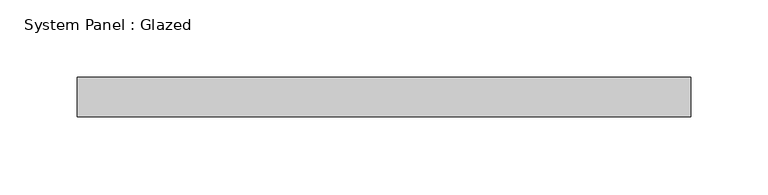
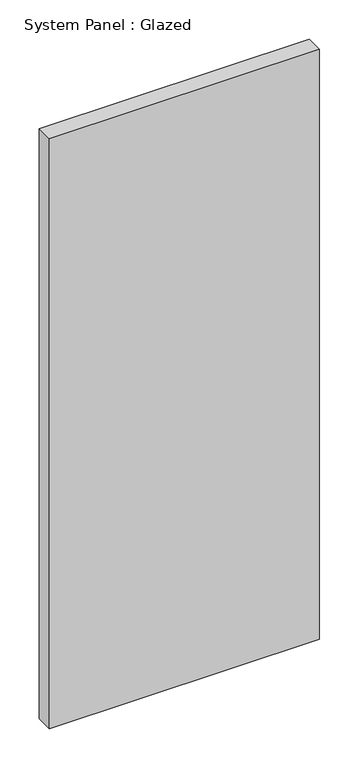
"""IFC4 building model written with IfcOpenShell, lengths in millimetres: plate geometry, System Panel : Glazed."""

from ifc_helpers import new_model, si_unit, origin, origin_with_axes, place, context, project, spatial, polyline, outline, extrude, source, transform, mapped, element, save


def system_panel_glazed_309beea3(model_context):
    return source(origin(), model_context, "Body", "SweptSolid", [
        extrude(outline(polyline([(197.8298794, 19.05), (-197.8298794, 19.05), (-197.8298794, 44.45), (197.8298794, 44.45), (197.8298794, 19.05)])), origin_with_axes(), (0.0, 0.0, 1.0), 914.4),
    ])


if __name__ == "__main__":
    model = new_model("IFC4")
    model_context = context("Model", 3, world=origin())
    ifc_project = project(units=[si_unit("LENGTHUNIT", "METRE", prefix="MILLI")], contexts=[model_context])
    site = spatial("IfcSite", under=ifc_project)
    building = spatial("IfcBuilding", under=site)
    placement = place(None, origin())
    system_panel_glazed_shape = system_panel_glazed_309beea3(model_context)
    element("IfcPlate", 1, ObjectType="System Panel : Glazed", at=placement, inside=building, context=model_context, shape_type="MappedRepresentation", body=[
        mapped(system_panel_glazed_shape, transform((0.0, 0.0, 0.0), x_axis=(1.0, 0.0, 0.0), y_axis=(0.0, 1.0, 0.0), z_axis=(0.0, 0.0, 1.0))),
    ])
    save(model, "model.ifc")

# Revit data of these elements
# Type "System Panel : Glazed"
#   Construction Type Id = "GSP4R"
#   Analytic Construction = "1/8 in Pilkington single glazing"
#   Visual Light Transmittance = 0.9
#   Solar Heat Gain Coefficient = 0.86
#   Heat Transfer Coefficient (U) = 1.18115 BTU/(h·ft²·°F)
# Element 1 (IfcPlate, "System Panel : Glazed")
#   Materials on its faces: "Glass"
# Materials
#   "Glass": class "Glass", colour RGB 0 128 192, transparency 0.75, Description = "Soda Lime Glass", Cost = 0
